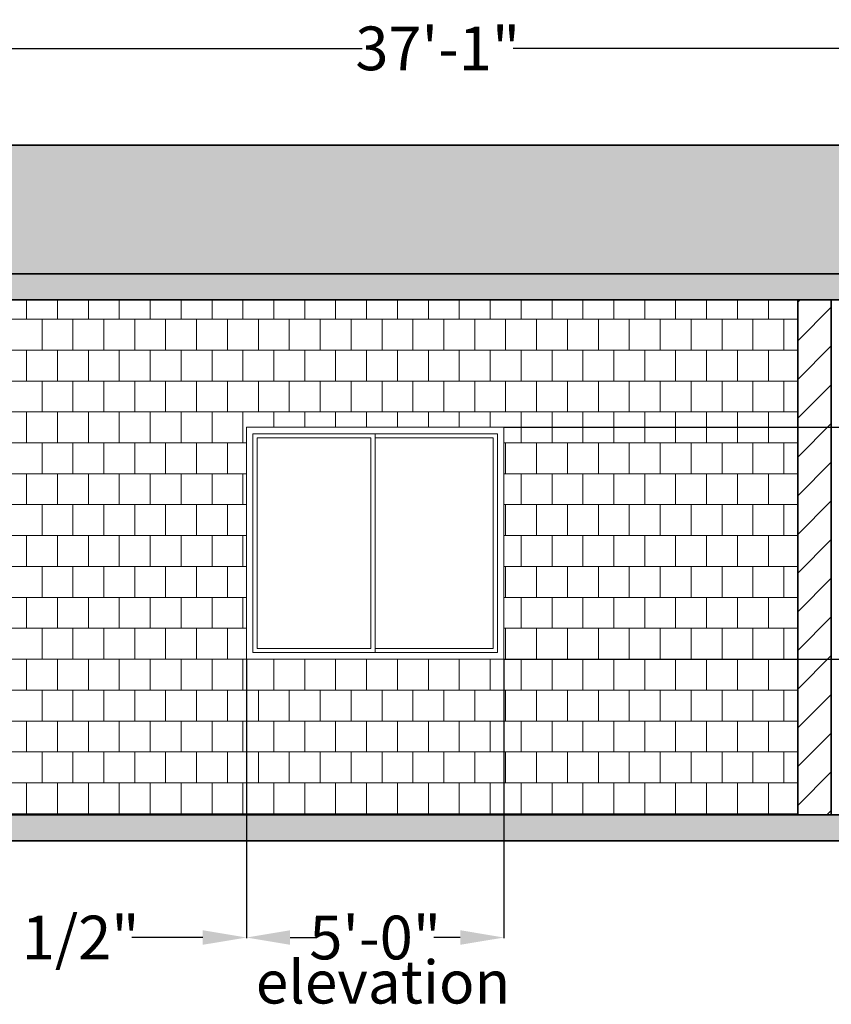
# Model space of a CAD drawing. Units: inches. Extents: x 1222 to 2611, y 176 to 793.
# Tile 4 of 5: x 1746 to 1935, y 526 to 755. Entities that reach past the tile are written whole.
import ezdxf

# ---------------------------------------------------------------- set-up
doc = ezdxf.new("R2010")
doc.units = ezdxf.units.IN
doc.header["$MEASUREMENT"] = 0
for name, color, linetype, lineweight in [('A-ANNO-DIMS', 2, 'Continuous', 18), ('A-ANNO-TEXT', 7, 'Continuous', 25), ('A-ELEV', 7, 'Continuous', 35), ('A-ELEV-GLAZ', 4, 'Continuous', 18), ('A-ELEV-PATT', 30, 'Continuous', 13)]:
    doc.layers.add(name, color=color, linetype=linetype, lineweight=lineweight)
doc.styles.get("Standard").update_dxf_attribs({"font": 'arial.ttf'})
doc.dimstyles.get("Standard").update_dxf_attribs({"dimtxt": 10.18, "dimasz": 10.18, "dimexe": 0.18, "dimexo": 0.0625, "dimgap": 0.09, "dimtad": 0, "dimtih": 1, "dimtoh": 1, "dimdec": 0, "dimzin": 0, "dimdsep": 46, "dimlunit": 3, "dimtxsty": 'Standard', "dimcen": 0.09, "dimadec": 0, "dimazin": 0, "dimtfac": 1, "dimtdec": 0, "dimtofl": 0, "dimtmove": 0, "dimatfit": 3, "dimfxl": 1, "dimtolj": 1, "dimtzin": 0, "dimarcsym": 0})

# ---------------------------------------------------------------- blocks, each defined once
blk = doc.blocks.new('*U7')
for p, q in [((1.5, 1.5), (1.5, 52.5)), ((1.5, 52.5), (30, 52.5)), ((30, 1.5), (30, 52.5)), ((30, 52.5), (58.5, 52.5)), ((58.5, 52.5), (58.5, 1.5)), ((30, 1.5), (1.5, 1.5)), ((58.5, 1.5), (30, 1.5))]:
    blk.add_line(p, q)
blk.add_lwpolyline([(0, 0), (0, 54), (60, 54), (60, 0)], close=True)
for points in [[(29, 51.5), (29, 2.5), (2.5, 2.5), (2.5, 51.5), (29, 51.5)], [(30, 51.5), (57.5, 51.5), (57.5, 2.5), (30, 2.5)]]:
    blk.add_lwpolyline(points)
blk = doc.blocks.new('*D42')
at = {"layer": 'A-ANNO-DIMS', "color": 0, "lineweight": -2, "transparency": 16777216}
for p, q in [((1620.56, 726.3), (1620.56, 748.97)), ((1630.74, 748.79), (1825.48, 748.79)), ((2055.37, 748.79), (1860.63, 748.79)), ((2065.55, 726.3), (2065.55, 748.97))]:
    blk.add_line(p, q, dxfattribs=at)
at = {"layer": 'A-ANNO-DIMS', "color": 0, "transparency": 16777216}
for points in [[(1630.74, 750.49), (1630.74, 747.1), (1620.56, 748.79)], [(2055.37, 750.49), (2055.37, 747.1), (2065.55, 748.79)]]:
    blk.add_solid(points, dxfattribs=at)
at = {"layer": 'Defpoints', "color": 0, "transparency": 16777216}
for p in [(2065.55, 748.79), (1620.56, 726.24), (2065.55, 726.24)]:
    blk.add_point(p, dxfattribs=at)
at = {"layer": 'A-ANNO-DIMS', "color": 0, "transparency": 16777216, "insert": (1843.06, 748.79), "char_height": 10.18, "attachment_point": 5}
blk.add_mtext('\\A1;37\'-1"', dxfattribs=at)
blk = doc.blocks.new('*D50')
at = {"layer": 'A-ANNO-DIMS', "color": 0, "lineweight": -2, "transparency": 16777216}
for p, q in [((1798.49, 606.49), (1798.49, 541.51)), ((1694.04, 603.54), (1694.04, 541.51)), ((1704.22, 541.69), (1720.78, 541.69)), ((1788.31, 541.69), (1771.76, 541.69))]:
    blk.add_line(p, q, dxfattribs=at)
at = {"layer": 'A-ANNO-DIMS', "color": 0, "transparency": 16777216}
for points in [[(1704.22, 543.39), (1704.22, 540), (1694.04, 541.69)], [(1788.31, 543.39), (1788.31, 540), (1798.49, 541.69)]]:
    blk.add_solid(points, dxfattribs=at)
at = {"layer": 'Defpoints', "color": 0, "transparency": 16777216}
for p in [(1798.49, 606.55), (1694.04, 603.6), (1798.49, 541.69)]:
    blk.add_point(p, dxfattribs=at)
at = {"layer": 'A-ANNO-DIMS', "color": 0, "transparency": 16777216, "insert": (1746.27, 541.69), "char_height": 10.18, "attachment_point": 5}
blk.add_mtext('\\A1;8\'-8 1/2"', dxfattribs=at)
blk = doc.blocks.new('*D51')
at = {"layer": 'A-ANNO-DIMS', "color": 0, "lineweight": -2, "transparency": 16777216}
for p, q in [((1798.49, 606.49), (1798.49, 541.51)), ((1858.49, 606.49), (1858.49, 541.51)), ((1808.67, 541.69), (1814.87, 541.69)), ((1848.31, 541.69), (1842.11, 541.69))]:
    blk.add_line(p, q, dxfattribs=at)
at = {"layer": 'A-ANNO-DIMS', "color": 0, "transparency": 16777216}
for points in [[(1808.67, 543.39), (1808.67, 540), (1798.49, 541.69)], [(1848.31, 543.39), (1848.31, 540), (1858.49, 541.69)]]:
    blk.add_solid(points, dxfattribs=at)
at = {"layer": 'Defpoints', "color": 0, "transparency": 16777216}
for p in [(1798.49, 606.55), (1858.49, 606.55), (1858.49, 541.69)]:
    blk.add_point(p, dxfattribs=at)
at = {"layer": 'A-ANNO-DIMS', "color": 0, "transparency": 16777216, "insert": (1828.49, 541.69), "char_height": 10.18, "attachment_point": 5}
blk.add_mtext('\\A1;5\'-0"', dxfattribs=at)
blk = doc.blocks.new('*D54')
at = {"layer": 'A-ANNO-DIMS', "color": 0, "lineweight": -2, "transparency": 16777216}
for p, q in [((1858.56, 660.55), (2088.95, 660.55)), ((2088.77, 650.37), (2088.77, 638.84)), ((2088.77, 616.73), (2088.77, 628.26)), ((1858.56, 606.55), (2088.95, 606.55))]:
    blk.add_line(p, q, dxfattribs=at)
at = {"layer": 'A-ANNO-DIMS', "color": 0, "transparency": 16777216}
for points in [[(2087.07, 650.37), (2090.47, 650.37), (2088.77, 660.55)], [(2087.07, 616.73), (2090.47, 616.73), (2088.77, 606.55)]]:
    blk.add_solid(points, dxfattribs=at)
at = {"layer": 'Defpoints', "color": 0, "transparency": 16777216}
for p in [(1858.49, 660.55), (2088.77, 660.55), (1858.49, 606.55)]:
    blk.add_point(p, dxfattribs=at)
at = {"layer": 'A-ANNO-DIMS', "color": 0, "transparency": 16777216, "insert": (2088.77, 633.55), "char_height": 10.18, "attachment_point": 5}
blk.add_mtext('\\A1;4\'-6"', dxfattribs=at)
blk = doc.blocks.new('*D55')
at = {"layer": 'A-ANNO-DIMS', "color": 0, "lineweight": -2, "transparency": 16777216}
for p, q in [((1858.56, 606.55), (2088.95, 606.55)), ((2088.77, 596.37), (2088.77, 593.75)), ((2088.77, 580.42), (2088.77, 583.04)), ((1926.97, 570.24), (2088.95, 570.24))]:
    blk.add_line(p, q, dxfattribs=at)
at = {"layer": 'A-ANNO-DIMS', "color": 0, "transparency": 16777216}
for points in [[(2087.07, 596.37), (2090.47, 596.37), (2088.77, 606.55)], [(2087.07, 580.42), (2090.47, 580.42), (2088.77, 570.24)]]:
    blk.add_solid(points, dxfattribs=at)
at = {"layer": 'Defpoints', "color": 0, "transparency": 16777216}
for p in [(1858.49, 606.55), (2088.77, 606.55), (1926.91, 570.24)]:
    blk.add_point(p, dxfattribs=at)
at = {"layer": 'A-ANNO-DIMS', "color": 0, "transparency": 16777216, "insert": (2088.77, 588.4), "char_height": 10.18, "attachment_point": 5}
blk.add_mtext('\\A1;3\'-0 1/2"', dxfattribs=at)

msp = doc.modelspace()

# ---------------------------------------------------------------- hatches: boundary and pattern name
at = {"layer": 'A-ELEV-PATT'}
h = msp.add_hatch(dxfattribs=at)
h.set_pattern_fill('AR-BRSTD', color=256, scale=0.9)
h.set_pattern_definition([(0, (-599.9298, -178.2906), (0, 2.4003), []), (90, (-599.9298, -178.2906), (-3.6, 2.4003), [2.4003, -2.4003])])
h.paths.add_polyline_path([(2065.55, 696.24), (2065.55, 726.24), (1629.56, 726.24), (1629.56, 696.24)])
h = msp.add_hatch(dxfattribs=at)
h.set_pattern_fill('AR-CONC', color=256, scale=0.9)
h.set_pattern_definition([(50, (-599.93, -178.2906), (6.455342, -0.564769), [0.675, -7.425]), (355, (-599.93, -178.2906), (-1.248762, 6.769729), [0.54, -5.94]), (100.45144, (-599.392, -178.3376), (5.20658, 6.20496), [0.573662, -6.310279]), (46.1842, (-599.93, -176.4906), (9.605172, -1.489674), [1.0125, -11.1375]), (96.63564, (-599.129, -176.615), (8.411958, 8.767067), [0.860493, -9.465424]), (351.18416, (-599.93, -176.491), (8.411958, 8.767067), [0.81, -8.91]), (21, (-599.03, -176.9406), (5.372163, -3.62357), [0.675, -7.425]), (326, (-599.03, -176.9406), (2.189838, 6.52635), [0.54, -5.94]), (71.45144, (-598.582, -177.2425), (7.562001, 2.90278), [0.573662, -6.310279]), (37.5, (-599.9298, -178.2906), (0.1094387, 2.9960447), [0, -5.868, 0, -6.03, 0, -5.9625]), (7.5, (-599.9298, -178.2906), (2.367626, 3.5497054), [0, -3.438, 0, -5.733, 0, -2.2725]), (327.5, (-601.9368, -178.2906), (4.804402, -0.2029938), [0, -2.25, 0, -7.02, 0, -9.315]), (317.5, (-602.837, -178.2906), (5.2486755, 0.900945), [0, -2.925, 0, -4.662, 0, -6.615])])
h.paths.add_polyline_path([(1926.91, 690.24), (2065.55, 690.24), (2065.55, 696.24), (1629.56, 696.24), (1629.56, 690.24)])
h.paths.add_polyline_path([(1629.56, 570.24), (1629.56, 564.24), (2065.55, 564.24), (2065.55, 570.24), (2007.5, 570.24), (2006.95, 569.97), (2006.81, 570.24)])
h = msp.add_hatch(dxfattribs=at)
h.set_pattern_fill('ANSI31', color=256, scale=51)
h.set_pattern_definition([(45, (-599.93, -178.2906), (-4.507806, 4.507806), [])])
h.paths.add_polyline_path([(1629.56, 690.24), (1620.56, 690.24), (1620.56, 570.24), (1629.56, 570.24)])
h.paths.add_polyline_path([(1934.74, 690.24), (1926.91, 690.24), (1926.91, 570.24), (1934.74, 570.24)])
h = msp.add_hatch(dxfattribs=at)
h.set_pattern_fill('AR-B88', color=256, scale=0.9)
h.set_pattern_definition([(0, (-599.93, -178.2906), (0, 7.2), []), (90, (-599.9298, -178.2906), (-3.6, 7.2), [7.2, -7.2])])
h.paths.add_polyline_path([(1629.56, 690.24), (1629.56, 570.24), (1926.91, 570.24), (1926.91, 690.24)])
h.paths.add_polyline_path([(1798.49, 660.55), (1858.49, 660.55), (1858.49, 606.55), (1798.49, 606.55)], flags=16)
h.paths.add_polyline_path([(1799.99, 659.05), (1828.49, 659.05), (1856.99, 659.05), (1856.99, 608.05), (1828.49, 608.05), (1799.99, 608.05)], flags=0)
h.paths.add_polyline_path([(1827.49, 609.05), (1827.49, 658.05), (1800.99, 658.05), (1800.99, 609.05)], flags=0)
h.paths.add_polyline_path([(1694.04, 639.6), (1694.04, 603.6), (1658.04, 603.6), (1658.04, 639.6)], flags=16)
h.paths.add_polyline_path([(1692.54, 638.1), (1692.54, 605.1), (1676.04, 605.1), (1659.54, 605.1), (1659.54, 638.1), (1676.04, 638.1)], flags=0)
h.paths.add_polyline_path([(1675.04, 606.1), (1675.04, 637.1), (1660.54, 637.1), (1660.54, 606.1)], flags=0)
h.paths.add_polyline_path([(1828.49, 658.05), (1855.99, 658.05), (1855.99, 609.05), (1828.49, 609.05)], flags=0)
h.paths.add_polyline_path([(1691.54, 637.1), (1691.54, 606.1), (1676.04, 606.1), (1676.04, 637.1)], flags=0)
h = msp.add_hatch(dxfattribs=at)
h.set_pattern_fill('GRAVEL', color=256, scale=1.6)
h.set_pattern_definition([(228.0127875, (-598.7778, -176.69058), (-12.8, -14.4), [0.2152576, -21.3105409]), (184.9697407, (-598.921794, -176.850575), (19.2, 1.6), [0.3693888, -36.5694796]), (132.510447, (-599.28979, -176.882575), (16, -17.6), [0.2604608, -25.78565215]), (267.273689, (-599.913794, -177.282575), (1.6, 32), [0.3363808, -33.3016929]), (292.8336542, (-599.929794, -177.618575), (-8, 19.2), [0.329848, -32.654997]), (357.273689, (-599.801794, -177.922575), (-32, 1.6), [0.3363808, -33.3016929]), (37.6942405, (-599.465794, -177.938575), (-20.8, -16), [0.4448464, -44.0397577]), (72.2553284, (-599.113794, -177.666575), (11.2, 35.2), [0.4199808, -41.5781144]), (121.4295656, (-598.985794, -177.266575), (-12.8, 20.8), [0.33752, -33.414517]), (175.2363583, (-599.1618, -176.97858), (17.6, -1.6), [0.3853312, -18.8812201]), (222.3974378, (-599.545794, -176.946575), (-19.2, -17.6), [0.4983168, -49.3334]), (138.814075, (-598.3298, -177.29858), (-11.2, 9.6), [0.1700816, -16.8381517]), (171.4692344, (-598.457794, -177.186575), (20.8, -3.2), [0.3235792, -32.0344183]), (225, (-598.7778, -177.1386), (-2e-16, -1.6), [0.2262736, -2.0364681]), (203.1985905, (-598.8898, -176.94658), (8, 3.2), [0.1218528, -12.0633842]), (291.80141, (-599.0018, -176.99458), (-1.6, 4.8), [0.1723248, -8.4439389]), (30.963757, (-598.9378, -177.15458), (4.8, 3.2), [0.2798864, -9.0496366]), (161.565051, (-598.6978, -177.0106), (3.2, -1.6), [0.2023856, -4.8572587]), (16.3895403, (-599.92979, -176.994575), (16, 4.8), [0.28352, -28.0685522]), (70.346176, (-599.65779, -176.91458), (-6.4, -17.6), [0.2378576, -23.5478524]), (293.1985905, (-598.6978, -176.69058), (-3.2, 8), [0.243704, -11.941533]), (343.6104597, (-598.60179, -176.914575), (-16, 4.8), [0.28352, -28.0685522]), (339.443955, (-599.9298, -177.98658), (-8, 3.2), [0.273408, -13.396998]), (294.7751406, (-599.67379, -178.08258), (-8, 17.6), [0.2290848, -22.6794289]), (66.8014095, (-598.6818, -178.29058), (3.2, 8), [0.243704, -11.941533]), (17.3540246, (-598.58579, -178.066575), (-20.8, -6.4), [0.2682096, -26.5526778]), (69.443955, (-599.4658, -178.29058), (-3.2, -8), [0.136704, -13.533702]), (101.309932, (-598.7778, -178.29058), (-1.6, 6.4), [0.081584, -8.0768472]), (165.963757, (-598.7938, -178.21058), (4.8, -1.6), [0.329848, -6.267121]), (186.009006, (-599.113794, -178.130575), (16, 1.6), [0.30568, -30.2622771]), (303.690068, (-598.9378, -177.29858), (-1.6, 3.2), [0.2307552, -5.5381268]), (353.1572266, (-598.809794, -177.490575), (27.2, -3.2), [0.4028704, -39.8841002]), (60.945396, (-598.4098, -177.53858), (-6.4, -11.2), [0.1647296, -16.3082786]), (90, (-598.3298, -177.3946), (-1.6, 1.6), [0.096, -1.504]), (120.256437, (-599.14579, -178.08258), (6.4, -11.2), [0.2222784, -22.005632]), (48.0127875, (-599.2578, -177.89058), (12.8, 14.4), [0.4305152, -21.0952833]), (0, (-598.9698, -177.5706), (1.6, 1.6), [0.416, -1.184]), (325.3048465, (-598.55379, -177.57058), (16, -11.2), [0.2529824, -25.0452389]), (254.054604, (-598.3458, -177.71458), (-1.6, -6.4), [0.2329632, -11.4152126]), (207.6459754, (-598.409794, -177.938575), (-30.4, -16), [0.379304, -37.5511587]), (175.4260787, (-598.745794, -178.114575), (-20.8, 1.6), [0.4012784, -39.72651745])])
edge = h.paths.add_edge_path(flags=17)
edge.add_line((2065.55, 690.24), (1934.74, 690.24))
edge.add_line((1934.74, 690.24), (1934.74, 570.24))
edge.add_line((1934.74, 570.24), (1963.73, 570.24))
edge.add_line((1963.73, 570.24), (1963.88, 571.16))
edge.add_line((1963.88, 571.16), (1963.88, 572.07))
edge.add_line((1963.88, 572.07), (1963.06, 572.64))
edge.add_line((1963.06, 572.64), (1963.25, 572.73))
edge.add_line((1963.25, 572.73), (1962.23, 573.02))
edge.add_line((1962.23, 573.02), (1962.34, 573.13))
edge.add_line((1962.34, 573.13), (1961.94, 573.08))
edge.add_line((1961.94, 573.08), (1962.03, 573.77))
edge.add_line((1962.03, 573.77), (1961.67, 573.89))
edge.add_line((1961.67, 573.89), (1961.59, 574.79))
edge.add_line((1961.59, 574.79), (1961.58, 574.81))
edge.add_line((1961.58, 574.81), (1961.4, 574.75))
edge.add_line((1961.4, 574.75), (1961.49, 575.28))
edge.add_line((1961.49, 575.28), (1961.16, 576.33))
edge.add_line((1961.16, 576.33), (1961.25, 577.97))
edge.add_line((1961.25, 577.97), (1961.22, 577.99))
edge.add_line((1961.22, 577.99), (1961.71, 578.69))
edge.add_line((1961.71, 578.69), (1961.35, 578.57))
edge.add_line((1961.35, 578.57), (1961.62, 578.98))
edge.add_line((1961.62, 578.98), (1961.71, 579.56))
edge.add_line((1961.71, 579.56), (1961.58, 579.67))
edge.add_line((1961.58, 579.67), (1962.11, 580.92))
edge.add_line((1962.11, 580.92), (1962.12, 580.83))
edge.add_line((1962.12, 580.83), (1962.34, 581.23))
edge.add_line((1962.34, 581.23), (1962.61, 581.29))
edge.add_line((1962.61, 581.29), (1962.75, 582.05))
edge.add_line((1962.75, 582.05), (1962.43, 582.39))
edge.add_line((1962.43, 582.39), (1962.7, 582.62))
edge.add_line((1962.7, 582.62), (1963.34, 583.37))
edge.add_line((1963.34, 583.37), (1963.21, 584.02))
edge.add_line((1963.21, 584.02), (1963.88, 584.59))
edge.add_line((1963.88, 584.59), (1964.19, 585.28))
edge.add_line((1964.19, 585.28), (1964.37, 584.82))
edge.add_line((1964.37, 584.82), (1964.46, 584.94))
edge.add_line((1964.46, 584.94), (1964.74, 584.18))
edge.add_line((1964.74, 584.18), (1964.87, 584.3))
edge.add_line((1964.87, 584.3), (1965.23, 583.37))
edge.add_line((1965.23, 583.37), (1965.37, 583.61))
edge.add_line((1965.37, 583.61), (1965.68, 582.97))
edge.add_line((1965.68, 582.97), (1965.55, 582.28))
edge.add_line((1965.55, 582.28), (1965.95, 582.16))
edge.add_line((1965.95, 582.16), (1966.25, 581.03))
edge.add_line((1966.25, 581.03), (1966.18, 581.06))
edge.add_line((1966.18, 581.06), (1966.38, 579.5))
edge.add_line((1966.38, 579.5), (1966.58, 579.47))
edge.add_line((1966.58, 579.47), (1966.27, 578.92))
edge.add_line((1966.27, 578.92), (1966.63, 578.69))
edge.add_line((1966.63, 578.69), (1966.41, 578.48))
edge.add_line((1966.41, 578.48), (1967.13, 577.3))
edge.add_line((1967.13, 577.3), (1966.81, 576.14))
edge.add_line((1966.81, 576.14), (1967.22, 575.18))
edge.add_line((1967.22, 575.18), (1966.4, 574.7))
edge.add_line((1966.4, 574.7), (1966.81, 574.47))
edge.add_line((1966.81, 574.47), (1966.77, 574))
edge.add_line((1966.77, 574), (1966.27, 573.77))
edge.add_line((1966.27, 573.77), (1965.95, 573.31))
edge.add_line((1965.95, 573.31), (1966.09, 572.96))
edge.add_line((1966.09, 572.96), (1965.37, 572.38))
edge.add_line((1965.37, 572.38), (1965.32, 572.21))
edge.add_line((1965.32, 572.21), (1965.05, 572.32))
edge.add_line((1965.05, 572.32), (1964.43, 572.04))
edge.add_line((1964.43, 572.04), (1964.36, 571.28))
edge.add_line((1964.36, 571.28), (1964.36, 570.53))
edge.add_line((1964.36, 570.53), (1964.41, 570.24))
edge.add_line((1964.41, 570.24), (1987.91, 570.24))
edge.add_line((1987.91, 570.24), (1996.3, 582.56))
edge.add_line((1996.3, 582.56), (1987.54, 582.59))
edge.add_spline(control_points=[(1987.95, 582.58), (1987.69, 582.31), (1986.78, 583.07), (1985.86, 583.82)], knot_values=[0, 0, 0, 0, 1.984581, 1.984581, 1.984581, 1.984581], degree=3, periodic=0)
edge.add_line((1985.86, 583.82), (1985.86, 584.58))
edge.add_line((1985.86, 584.58), (1983.48, 584.58))
edge.add_line((1983.48, 584.58), (1983.48, 586.08))
edge.add_line((1983.48, 586.08), (2015.16, 586.08))
edge.add_line((2015.16, 586.08), (2015.16, 584.58))
edge.add_line((2015.16, 584.58), (2012.63, 584.58))
edge.add_line((2012.63, 584.58), (2012.63, 583.56))
edge.add_spline(control_points=[(2012.63, 583.56), (2012.63, 583.55), (2012.63, 583.54), (2012.63, 583.53)], knot_values=[1.450992, 1.450992, 1.450992, 1.450992, 1.529987, 1.529987, 1.529987, 1.529987], degree=3, periodic=0)
edge.add_spline(control_points=[(2012.63, 583.53), (2012.58, 583.36), (2011.76, 582.94), (2010.94, 582.53)], knot_values=[0, 0, 0, 0, 1.450992, 1.450992, 1.450992, 1.450992], degree=3, periodic=0)
edge.add_line((2010.94, 582.53), (2000.52, 582.55))
edge.add_line((2000.52, 582.55), (2006.81, 570.24))
edge.add_line((2006.81, 570.24), (2020.56, 570.24))
edge.add_line((2020.56, 570.24), (2020.56, 571.2))
edge.add_arc((2020.56, 573.26), 2.06, 180, 270, ccw=False)
edge.add_spline(control_points=[(2018.51, 573.26), (2017.72, 573.63), (2017.98, 574.82), (2018.24, 576.02)], knot_values=[0, 0, 0, 0, 2.696371, 2.696371, 2.696371, 2.696371], degree=3, periodic=0)
edge.add_line((2018.24, 576.02), (2017.97, 576.02))
edge.add_line((2017.97, 576.02), (2017.97, 578.04))
edge.add_line((2017.97, 578.04), (2018.51, 586.16))
edge.add_arc((2020.56, 586.16), 2.06, 90, 180, ccw=False)
edge.add_line((2020.56, 588.21), (2032.66, 588.21))
edge.add_spline(control_points=[(2032.66, 588.21), (2032.66, 588.37), (2032.61, 589.89), (2033.94, 591.39), (2035.47, 592.42)], knot_values=[9.985388, 9.985388, 9.985388, 9.985388, 10.44542, 14.413405, 14.413405, 14.413405, 14.413405], degree=3, periodic=0)
edge.add_spline(control_points=[(2035.47, 592.42), (2038.05, 594.16), (2043.35, 595.42), (2042.75, 591.42), (2042.55, 590.1)], knot_values=[0, 0, 0, 0, 6.689787, 9.985388, 9.985388, 9.985388, 9.985388], degree=3, periodic=0)
edge.add_line((2042.55, 590.1), (2042.23, 586.16))
edge.add_line((2042.23, 586.16), (2042.23, 573.26))
edge.add_arc((2040.17, 573.26), 2.06, -73.742, 0, ccw=False)
edge.add_line((2040.75, 571.29), (2040.75, 570.24))
edge.add_line((2040.75, 570.24), (2059.68, 570.24))
edge.add_line((2059.68, 570.24), (2059.82, 571.16))
edge.add_line((2059.82, 571.16), (2059.82, 572.07))
edge.add_line((2059.82, 572.07), (2059.01, 572.64))
edge.add_line((2059.01, 572.64), (2059.19, 572.73))
edge.add_line((2059.19, 572.73), (2058.17, 573.02))
edge.add_line((2058.17, 573.02), (2058.29, 573.13))
edge.add_line((2058.29, 573.13), (2057.88, 573.08))
edge.add_line((2057.88, 573.08), (2057.97, 573.77))
edge.add_line((2057.97, 573.77), (2057.61, 573.89))
edge.add_line((2057.61, 573.89), (2057.53, 574.79))
edge.add_line((2057.53, 574.79), (2057.52, 574.81))
edge.add_line((2057.52, 574.81), (2057.34, 574.75))
edge.add_line((2057.34, 574.75), (2057.43, 575.28))
edge.add_line((2057.43, 575.28), (2057.1, 576.33))
edge.add_line((2057.1, 576.33), (2057.19, 577.97))
edge.add_line((2057.19, 577.97), (2057.16, 577.99))
edge.add_line((2057.16, 577.99), (2057.65, 578.69))
edge.add_line((2057.65, 578.69), (2057.29, 578.57))
edge.add_line((2057.29, 578.57), (2057.56, 578.98))
edge.add_line((2057.56, 578.98), (2057.65, 579.56))
edge.add_line((2057.65, 579.56), (2057.52, 579.67))
edge.add_line((2057.52, 579.67), (2058.05, 580.92))
edge.add_line((2058.05, 580.92), (2058.06, 580.83))
edge.add_line((2058.06, 580.83), (2058.29, 581.23))
edge.add_line((2058.29, 581.23), (2058.56, 581.29))
edge.add_line((2058.56, 581.29), (2058.69, 582.05))
edge.add_line((2058.69, 582.05), (2058.38, 582.39))
edge.add_line((2058.38, 582.39), (2058.65, 582.62))
edge.add_line((2058.65, 582.62), (2059.28, 583.37))
edge.add_line((2059.28, 583.37), (2059.15, 584.02))
edge.add_line((2059.15, 584.02), (2059.82, 584.59))
edge.add_line((2059.82, 584.59), (2060.14, 585.28))
edge.add_line((2060.14, 585.28), (2060.32, 584.82))
edge.add_line((2060.32, 584.82), (2060.41, 584.94))
edge.add_line((2060.41, 584.94), (2060.68, 584.18))
edge.add_line((2060.68, 584.18), (2060.81, 584.3))
edge.add_line((2060.81, 584.3), (2061.17, 583.37))
edge.add_line((2061.17, 583.37), (2061.31, 583.61))
edge.add_line((2061.31, 583.61), (2061.63, 582.97))
edge.add_line((2061.63, 582.97), (2061.49, 582.28))
edge.add_line((2061.49, 582.28), (2061.9, 582.16))
edge.add_line((2061.9, 582.16), (2062.19, 581.03))
edge.add_line((2062.19, 581.03), (2062.12, 581.06))
edge.add_line((2062.12, 581.06), (2062.32, 579.5))
edge.add_line((2062.32, 579.5), (2062.52, 579.47))
edge.add_line((2062.52, 579.47), (2062.21, 578.92))
edge.add_line((2062.21, 578.92), (2062.57, 578.69))
edge.add_line((2062.57, 578.69), (2062.36, 578.48))
edge.add_line((2062.36, 578.48), (2063.07, 577.3))
edge.add_line((2063.07, 577.3), (2062.75, 576.14))
edge.add_line((2062.75, 576.14), (2063.16, 575.18))
edge.add_line((2063.16, 575.18), (2062.35, 574.7))
edge.add_line((2062.35, 574.7), (2062.75, 574.47))
edge.add_line((2062.75, 574.47), (2062.71, 574))
edge.add_line((2062.71, 574), (2062.21, 573.77))
edge.add_line((2062.21, 573.77), (2061.9, 573.31))
edge.add_line((2061.9, 573.31), (2062.03, 572.96))
edge.add_line((2062.03, 572.96), (2061.31, 572.38))
edge.add_line((2061.31, 572.38), (2061.26, 572.21))
edge.add_line((2061.26, 572.21), (2060.99, 572.32))
edge.add_line((2060.99, 572.32), (2060.38, 572.04))
edge.add_line((2060.38, 572.04), (2060.31, 571.28))
edge.add_line((2060.31, 571.28), (2060.31, 570.53))
edge.add_line((2060.31, 570.53), (2060.35, 570.24))
edge.add_line((2060.35, 570.24), (2065.55, 570.24))
edge.add_line((2065.55, 570.24), (2065.55, 690.24))
edge = h.paths.add_edge_path(flags=17)
edge.add_line((2065.55, 690.24), (1934.74, 690.24))
edge.add_line((1934.74, 690.24), (1934.74, 570.24))
edge.add_line((1934.74, 570.24), (1963.73, 570.24))
edge.add_line((1963.73, 570.24), (1963.88, 571.16))
edge.add_line((1963.88, 571.16), (1963.88, 572.07))
edge.add_line((1963.88, 572.07), (1963.43, 572.38))
edge.add_line((1963.43, 572.38), (1962.71, 572.88))
edge.add_line((1962.71, 572.88), (1962, 573.09))
edge.add_line((1962, 573.09), (1961.94, 573.08))
edge.add_line((1961.94, 573.08), (1962.03, 573.77))
edge.add_line((1962.03, 573.77), (1961.67, 573.89))
edge.add_line((1961.67, 573.89), (1961.59, 574.79))
edge.add_line((1961.59, 574.79), (1961.58, 574.81))
edge.add_line((1961.58, 574.81), (1961.4, 574.75))
edge.add_line((1961.4, 574.75), (1961.49, 575.28))
edge.add_line((1961.49, 575.28), (1961.31, 575.85))
edge.add_line((1961.31, 575.85), (1961.06, 576.63))
edge.add_line((1961.06, 576.63), (1961.17, 576.55))
edge.add_line((1961.17, 576.55), (1961.25, 577.97))
edge.add_line((1961.25, 577.97), (1961.22, 577.99))
edge.add_line((1961.22, 577.99), (1961.71, 578.69))
edge.add_line((1961.71, 578.69), (1961.35, 578.57))
edge.add_line((1961.35, 578.57), (1961.62, 578.98))
edge.add_line((1961.62, 578.98), (1961.71, 579.56))
edge.add_line((1961.71, 579.56), (1961.58, 579.67))
edge.add_line((1961.58, 579.67), (1961.85, 580.31))
edge.add_line((1961.85, 580.31), (1962.23, 581.21))
edge.add_line((1962.23, 581.21), (1962.61, 581.29))
edge.add_line((1962.61, 581.29), (1962.75, 582.05))
edge.add_line((1962.75, 582.05), (1962.43, 582.39))
edge.add_line((1962.43, 582.39), (1962.7, 582.62))
edge.add_line((1962.7, 582.62), (1963.34, 583.37))
edge.add_line((1963.34, 583.37), (1963.29, 583.61))
edge.add_line((1963.29, 583.61), (1963.21, 584.02))
edge.add_line((1963.21, 584.02), (1963.88, 584.59))
edge.add_line((1963.88, 584.59), (1964.19, 585.28))
edge.add_line((1964.19, 585.28), (1964.37, 584.82))
edge.add_line((1964.37, 584.82), (1964.46, 584.94))
edge.add_line((1964.46, 584.94), (1964.74, 584.18))
edge.add_line((1964.74, 584.18), (1964.87, 584.3))
edge.add_line((1964.87, 584.3), (1965.23, 583.37))
edge.add_line((1965.23, 583.37), (1965.37, 583.61))
edge.add_line((1965.37, 583.61), (1965.68, 582.97))
edge.add_line((1965.68, 582.97), (1965.55, 582.28))
edge.add_line((1965.55, 582.28), (1965.95, 582.16))
edge.add_line((1965.95, 582.16), (1966.18, 581.29))
edge.add_line((1966.18, 581.29), (1966.25, 581.03))
edge.add_line((1966.25, 581.03), (1966.18, 581.06))
edge.add_line((1966.18, 581.06), (1966.38, 579.5))
edge.add_line((1966.38, 579.5), (1966.4, 579.5))
edge.add_line((1966.4, 579.5), (1966.58, 579.47))
edge.add_line((1966.58, 579.47), (1966.27, 578.92))
edge.add_line((1966.27, 578.92), (1966.63, 578.69))
edge.add_line((1966.63, 578.69), (1966.41, 578.48))
edge.add_line((1966.41, 578.48), (1967.13, 577.3))
edge.add_line((1967.13, 577.3), (1966.81, 576.14))
edge.add_line((1966.81, 576.14), (1967.08, 575.51))
edge.add_line((1967.08, 575.51), (1967.22, 575.18))
edge.add_line((1967.22, 575.18), (1966.4, 574.7))
edge.add_line((1966.4, 574.7), (1966.81, 574.47))
edge.add_line((1966.81, 574.47), (1966.77, 574))
edge.add_line((1966.77, 574), (1966.27, 573.77))
edge.add_line((1966.27, 573.77), (1965.95, 573.31))
edge.add_line((1965.95, 573.31), (1966.09, 572.96))
edge.add_line((1966.09, 572.96), (1965.37, 572.38))
edge.add_line((1965.37, 572.38), (1965.32, 572.21))
edge.add_line((1965.32, 572.21), (1965.05, 572.32))
edge.add_line((1965.05, 572.32), (1964.43, 572.04))
edge.add_line((1964.43, 572.04), (1964.36, 571.28))
edge.add_line((1964.36, 571.28), (1964.36, 570.53))
edge.add_line((1964.36, 570.53), (1964.41, 570.24))
edge.add_line((1964.41, 570.24), (1987.91, 570.24))
edge.add_line((1987.91, 570.24), (1996.3, 582.56))
edge.add_line((1996.3, 582.56), (1987.95, 582.58))
edge.add_spline(control_points=[(1987.95, 582.58), (1987.87, 582.5), (1987.74, 582.51), (1987.56, 582.59)], knot_values=[1.393615, 1.393615, 1.393615, 1.393615, 1.984581, 1.984581, 1.984581, 1.984581], degree=3, periodic=0)
edge.add_spline(control_points=[(1987.56, 582.59), (1987.15, 582.76), (1986.5, 583.29), (1985.86, 583.82)], knot_values=[0, 0, 0, 0, 1.393615, 1.393615, 1.393615, 1.393615], degree=3, periodic=0)
edge.add_line((1985.86, 583.82), (1985.86, 584.58))
edge.add_line((1985.86, 584.58), (1983.48, 584.58))
edge.add_line((1983.48, 584.58), (1983.48, 586.08))
edge.add_line((1983.48, 586.08), (2015.16, 586.08))
edge.add_line((2015.16, 586.08), (2015.16, 584.58))
edge.add_line((2015.16, 584.58), (2012.63, 584.58))
edge.add_line((2012.63, 584.58), (2012.63, 583.56))
edge.add_spline(control_points=[(2012.63, 583.56), (2012.63, 583.55), (2012.63, 583.54), (2012.63, 583.53)], knot_values=[1.450992, 1.450992, 1.450992, 1.450992, 1.529987, 1.529987, 1.529987, 1.529987], degree=3, periodic=0)
edge.add_spline(control_points=[(2012.63, 583.53), (2012.58, 583.36), (2011.76, 582.94), (2010.94, 582.53)], knot_values=[0, 0, 0, 0, 1.450992, 1.450992, 1.450992, 1.450992], degree=3, periodic=0)
edge.add_line((2010.94, 582.53), (2000.52, 582.55))
edge.add_line((2000.52, 582.55), (2006.81, 570.24))
edge.add_line((2006.81, 570.24), (2020.56, 570.24))
edge.add_line((2020.56, 570.24), (2020.56, 571.2))
edge.add_arc((2020.56, 573.26), 2.06, 180, 270, ccw=False)
edge.add_spline(control_points=[(2018.51, 573.26), (2017.72, 573.63), (2017.98, 574.82), (2018.24, 576.02)], knot_values=[0, 0, 0, 0, 2.696371, 2.696371, 2.696371, 2.696371], degree=3, periodic=0)
edge.add_line((2018.24, 576.02), (2017.97, 576.02))
edge.add_line((2017.97, 576.02), (2017.97, 578.04))
edge.add_line((2017.97, 578.04), (2018.51, 586.16))
edge.add_arc((2020.56, 586.16), 2.06, 90, 180, ccw=False)
edge.add_line((2020.56, 588.21), (2032.66, 588.21))
edge.add_spline(control_points=[(2032.66, 588.21), (2032.66, 588.37), (2032.61, 589.89), (2033.94, 591.39), (2035.47, 592.42)], knot_values=[9.985388, 9.985388, 9.985388, 9.985388, 10.44542, 14.413405, 14.413405, 14.413405, 14.413405], degree=3, periodic=0)
edge.add_spline(control_points=[(2035.47, 592.42), (2038.05, 594.16), (2043.35, 595.42), (2042.75, 591.42), (2042.55, 590.1)], knot_values=[0, 0, 0, 0, 6.689787, 9.985388, 9.985388, 9.985388, 9.985388], degree=3, periodic=0)
edge.add_line((2042.55, 590.1), (2042.23, 586.16))
edge.add_line((2042.23, 586.16), (2042.23, 573.26))
edge.add_arc((2040.17, 573.26), 2.06, -73.742, 0, ccw=False)
edge.add_line((2040.75, 571.29), (2040.75, 570.24))
edge.add_line((2040.75, 570.24), (2059.68, 570.24))
edge.add_line((2059.68, 570.24), (2059.82, 571.16))
edge.add_line((2059.82, 571.16), (2059.82, 572.07))
edge.add_line((2059.82, 572.07), (2059.37, 572.38))
edge.add_line((2059.37, 572.38), (2058.66, 572.88))
edge.add_line((2058.66, 572.88), (2057.94, 573.09))
edge.add_line((2057.94, 573.09), (2057.88, 573.08))
edge.add_line((2057.88, 573.08), (2057.97, 573.77))
edge.add_line((2057.97, 573.77), (2057.61, 573.89))
edge.add_line((2057.61, 573.89), (2057.53, 574.79))
edge.add_line((2057.53, 574.79), (2057.52, 574.81))
edge.add_line((2057.52, 574.81), (2057.34, 574.75))
edge.add_line((2057.34, 574.75), (2057.43, 575.28))
edge.add_line((2057.43, 575.28), (2057.25, 575.85))
edge.add_line((2057.25, 575.85), (2057.01, 576.63))
edge.add_line((2057.01, 576.63), (2057.11, 576.55))
edge.add_line((2057.11, 576.55), (2057.19, 577.97))
edge.add_line((2057.19, 577.97), (2057.16, 577.99))
edge.add_line((2057.16, 577.99), (2057.65, 578.69))
edge.add_line((2057.65, 578.69), (2057.29, 578.57))
edge.add_line((2057.29, 578.57), (2057.56, 578.98))
edge.add_line((2057.56, 578.98), (2057.65, 579.56))
edge.add_line((2057.65, 579.56), (2057.52, 579.67))
edge.add_line((2057.52, 579.67), (2057.79, 580.31))
edge.add_line((2057.79, 580.31), (2058.17, 581.21))
edge.add_line((2058.17, 581.21), (2058.56, 581.29))
edge.add_line((2058.56, 581.29), (2058.69, 582.05))
edge.add_line((2058.69, 582.05), (2058.38, 582.39))
edge.add_line((2058.38, 582.39), (2058.65, 582.62))
edge.add_line((2058.65, 582.62), (2059.28, 583.37))
edge.add_line((2059.28, 583.37), (2059.23, 583.61))
edge.add_line((2059.23, 583.61), (2059.15, 584.02))
edge.add_line((2059.15, 584.02), (2059.82, 584.59))
edge.add_line((2059.82, 584.59), (2060.14, 585.28))
edge.add_line((2060.14, 585.28), (2060.32, 584.82))
edge.add_line((2060.32, 584.82), (2060.41, 584.94))
edge.add_line((2060.41, 584.94), (2060.68, 584.18))
edge.add_line((2060.68, 584.18), (2060.81, 584.3))
edge.add_line((2060.81, 584.3), (2061.17, 583.37))
edge.add_line((2061.17, 583.37), (2061.31, 583.61))
edge.add_line((2061.31, 583.61), (2061.63, 582.97))
edge.add_line((2061.63, 582.97), (2061.49, 582.28))
edge.add_line((2061.49, 582.28), (2061.9, 582.16))
edge.add_line((2061.9, 582.16), (2062.12, 581.29))
edge.add_line((2062.12, 581.29), (2062.19, 581.03))
edge.add_line((2062.19, 581.03), (2062.12, 581.06))
edge.add_line((2062.12, 581.06), (2062.32, 579.5))
edge.add_line((2062.32, 579.5), (2062.35, 579.5))
edge.add_line((2062.35, 579.5), (2062.52, 579.47))
edge.add_line((2062.52, 579.47), (2062.21, 578.92))
edge.add_line((2062.21, 578.92), (2062.57, 578.69))
edge.add_line((2062.57, 578.69), (2062.36, 578.48))
edge.add_line((2062.36, 578.48), (2063.07, 577.3))
edge.add_line((2063.07, 577.3), (2062.75, 576.14))
edge.add_line((2062.75, 576.14), (2063.02, 575.51))
edge.add_line((2063.02, 575.51), (2063.16, 575.18))
edge.add_line((2063.16, 575.18), (2062.35, 574.7))
edge.add_line((2062.35, 574.7), (2062.75, 574.47))
edge.add_line((2062.75, 574.47), (2062.71, 574))
edge.add_line((2062.71, 574), (2062.21, 573.77))
edge.add_line((2062.21, 573.77), (2061.9, 573.31))
edge.add_line((2061.9, 573.31), (2062.03, 572.96))
edge.add_line((2062.03, 572.96), (2061.31, 572.38))
edge.add_line((2061.31, 572.38), (2061.26, 572.21))
edge.add_line((2061.26, 572.21), (2060.99, 572.32))
edge.add_line((2060.99, 572.32), (2060.38, 572.04))
edge.add_line((2060.38, 572.04), (2060.31, 571.28))
edge.add_line((2060.31, 571.28), (2060.31, 570.53))
edge.add_line((2060.31, 570.53), (2060.35, 570.24))
edge.add_line((2060.35, 570.24), (2065.55, 570.24))
edge.add_line((2065.55, 570.24), (2065.55, 690.24))
h.paths.add_polyline_path([(2065.55, 690.24), (1934.74, 690.24), (1934.74, 570.24), (1963.73, 570.24), (1963.88, 571.16), (1963.88, 572.07), (1963.43, 572.38), (1962.71, 572.88), (1962, 573.09), (1961.94, 573.08), (1962.03, 573.77), (1961.67, 573.89), (1961.59, 574.79), (1961.58, 574.81), (1961.4, 574.75), (1961.49, 575.28), (1961.31, 575.85), (1961.06, 576.63), (1961.17, 576.55), (1961.25, 577.97), (1961.22, 577.99), (1961.71, 578.69), (1961.35, 578.57), (1961.62, 578.98), (1961.71, 579.56), (1961.58, 579.67), (1961.85, 580.31), (1962.23, 581.21), (1962.61, 581.29), (1962.75, 582.05), (1962.43, 582.39), (1962.7, 582.62), (1963.34, 583.37), (1963.29, 583.61), (1963.21, 584.02), (1963.88, 584.59), (1964.19, 585.28), (1964.37, 584.82), (1964.46, 584.94), (1964.74, 584.18), (1964.87, 584.3), (1965.23, 583.37), (1965.37, 583.61), (1965.68, 582.97), (1965.55, 582.28), (1965.95, 582.16), (1966.18, 581.29), (1966.25, 581.03), (1966.18, 581.06), (1966.38, 579.5), (1966.4, 579.5), (1966.58, 579.47), (1966.27, 578.92), (1966.63, 578.69), (1966.41, 578.48), (1967.13, 577.3), (1966.81, 576.14), (1967.08, 575.51), (1967.22, 575.18), (1966.4, 574.7), (1966.81, 574.47), (1966.77, 574), (1966.27, 573.77), (1965.95, 573.31), (1966.09, 572.96), (1965.37, 572.38), (1965.32, 572.21), (1965.05, 572.32), (1964.43, 572.04), (1964.36, 571.28), (1964.36, 570.53), (1964.41, 570.24), (1987.91, 570.24), (1996.3, 582.56), (2000.52, 582.55), (2006.81, 570.24), (2020.56, 570.24), (2020.56, 571.2, -0.414214), (2018.51, 573.26), (2018.51, 576.02), (2017.97, 576.02), (2017.97, 578.04), (2018.51, 586.16, -0.414214), (2020.56, 588.21), (2032.66, 588.21), (2040.17, 588.21, -0.414214), (2042.23, 586.16), (2042.23, 573.26, -0.333344), (2040.75, 571.29), (2040.75, 570.24), (2059.68, 570.24), (2059.82, 571.16), (2059.82, 572.07), (2059.37, 572.38), (2058.66, 572.88), (2057.94, 573.09), (2057.88, 573.08), (2057.97, 573.77), (2057.61, 573.89), (2057.53, 574.79), (2057.52, 574.81), (2057.34, 574.75), (2057.43, 575.28), (2057.25, 575.85), (2057.01, 576.63), (2057.11, 576.55), (2057.19, 577.97), (2057.16, 577.99), (2057.65, 578.69), (2057.29, 578.57), (2057.56, 578.98), (2057.65, 579.56), (2057.52, 579.67), (2057.79, 580.31), (2058.17, 581.21), (2058.56, 581.29), (2058.69, 582.05), (2058.38, 582.39), (2058.65, 582.62), (2059.28, 583.37), (2059.23, 583.61), (2059.15, 584.02), (2059.82, 584.59), (2060.14, 585.28), (2060.32, 584.82), (2060.41, 584.94), (2060.68, 584.18), (2060.81, 584.3), (2061.17, 583.37), (2061.31, 583.61), (2061.63, 582.97), (2061.49, 582.28), (2061.9, 582.16), (2062.12, 581.29), (2062.19, 581.03), (2062.12, 581.06), (2062.32, 579.5), (2062.35, 579.5), (2062.52, 579.47), (2062.21, 578.92), (2062.57, 578.69), (2062.36, 578.48), (2063.07, 577.3), (2062.75, 576.14), (2063.02, 575.51), (2063.16, 575.18), (2062.35, 574.7), (2062.75, 574.47), (2062.71, 574), (2062.21, 573.77), (2061.9, 573.31), (2062.03, 572.96), (2061.31, 572.38), (2061.26, 572.21), (2060.99, 572.32), (2060.38, 572.04), (2060.31, 571.28), (2060.31, 570.53), (2060.35, 570.24), (2065.55, 570.24)], flags=0)
edge = h.paths.add_edge_path(flags=0)
edge.add_line((1983.48, 586.08), (2015.16, 586.08))
edge.add_line((2015.16, 586.08), (2015.16, 584.58))
edge.add_line((2015.16, 584.58), (2012.63, 584.58))
edge.add_line((2012.63, 584.58), (2012.63, 583.56))
edge.add_spline(control_points=[(2012.63, 583.56), (2012.63, 583.55), (2012.63, 583.54), (2012.63, 583.53)], knot_values=[1.450992, 1.450992, 1.450992, 1.450992, 1.529987, 1.529987, 1.529987, 1.529987], degree=3, periodic=0)
edge.add_spline(control_points=[(2012.63, 583.53), (2012.58, 583.36), (2011.76, 582.94), (2010.94, 582.53)], knot_values=[0, 0, 0, 0, 1.450992, 1.450992, 1.450992, 1.450992], degree=3, periodic=0)
edge.add_line((2010.94, 582.53), (1987.95, 582.58))
edge.add_spline(control_points=[(1987.95, 582.58), (1987.69, 582.31), (1986.78, 583.07), (1985.86, 583.82)], knot_values=[0, 0, 0, 0, 1.984581, 1.984581, 1.984581, 1.984581], degree=3, periodic=0)
edge.add_line((1985.86, 583.82), (1985.86, 584.58))
edge.add_line((1985.86, 584.58), (1983.48, 584.58))
edge.add_line((1983.48, 584.58), (1983.48, 586.08))

# ---------------------------------------------------------------- linework, layer by layer
at = {"layer": 'A-ELEV'}
for p, q in [((1620.56, 726.24), (2065.55, 726.24)), ((1629.56, 696.24), (2065.55, 696.24)), ((1629.56, 690.24), (1926.91, 690.24)), ((1926.91, 570.24), (1926.91, 690.24)), ((1926.91, 690.24), (2065.55, 690.24)), ((1934.74, 570.24), (1934.74, 690.24)), ((1629.56, 570.24), (2065.55, 570.24)), ((1620.56, 564.24), (2065.55, 564.24))]:
    msp.add_line(p, q, dxfattribs=at)

# ---------------------------------------------------------------- block references
at = {"layer": 'A-ELEV-GLAZ'}
msp.add_blockref('*U7', (1798.49, 606.55), dxfattribs=at)

# ---------------------------------------------------------------- texts
at = {"layer": 'A-ANNO-TEXT', "insert": (1800.68, 536.32), "char_height": 10, "attachment_point": 1}
msp.add_mtext_dynamic_manual_height_columns('elevation', width=206.8442, gutter_width=1, heights=[0], dxfattribs=at)

# ---------------------------------------------------------------- dimensions: what is measured, and where the dimension line sits
at = {"layer": 'A-ANNO-DIMS'}
for base, p1, p2, picture, middle in [((2065.55, 748.79), (1620.56, 726.24), (2065.55, 726.24), '*D42', (1843.06, 748.79)), ((1798.4942, 541.6919), (1694.045, 603.6028), (1798.4942, 606.5482), '*D50', (1746.2696, 541.6919)), ((1858.49, 541.69), (1798.49, 606.55), (1858.49, 606.55), '*D51', (1828.49, 541.69))]:
    dim = msp.add_linear_dim(base=base, p1=p1, p2=p2, dimstyle='Standard', override={"dimdec": 1, "dimlfac": 1, "dimrnd": 0, "dimzin": 1, "dimdsep": 46, "dimlunit": 4, "dimfrac": 2}, dxfattribs=at)
    dim.commit()
    dim.dimension.update_dxf_attribs({"geometry": picture, "text_midpoint": middle})
for base, p1, p2, picture, middle in [((2088.77, 660.55), (1858.49, 606.55), (1858.49, 660.55), '*D54', (2088.77, 633.55)), ((2088.77, 606.55), (1926.91, 570.24), (1858.49, 606.55), '*D55', (2088.77, 588.4))]:
    dim = msp.add_linear_dim(base=base, p1=p1, p2=p2, angle=90, dimstyle='Standard', override={"dimdec": 1, "dimlfac": 1, "dimrnd": 0, "dimzin": 1, "dimdsep": 46, "dimlunit": 4, "dimfrac": 2}, dxfattribs=at)
    dim.commit()
    dim.dimension.update_dxf_attribs({"geometry": picture, "text_midpoint": middle})

doc.saveas('drawing.dxf')
